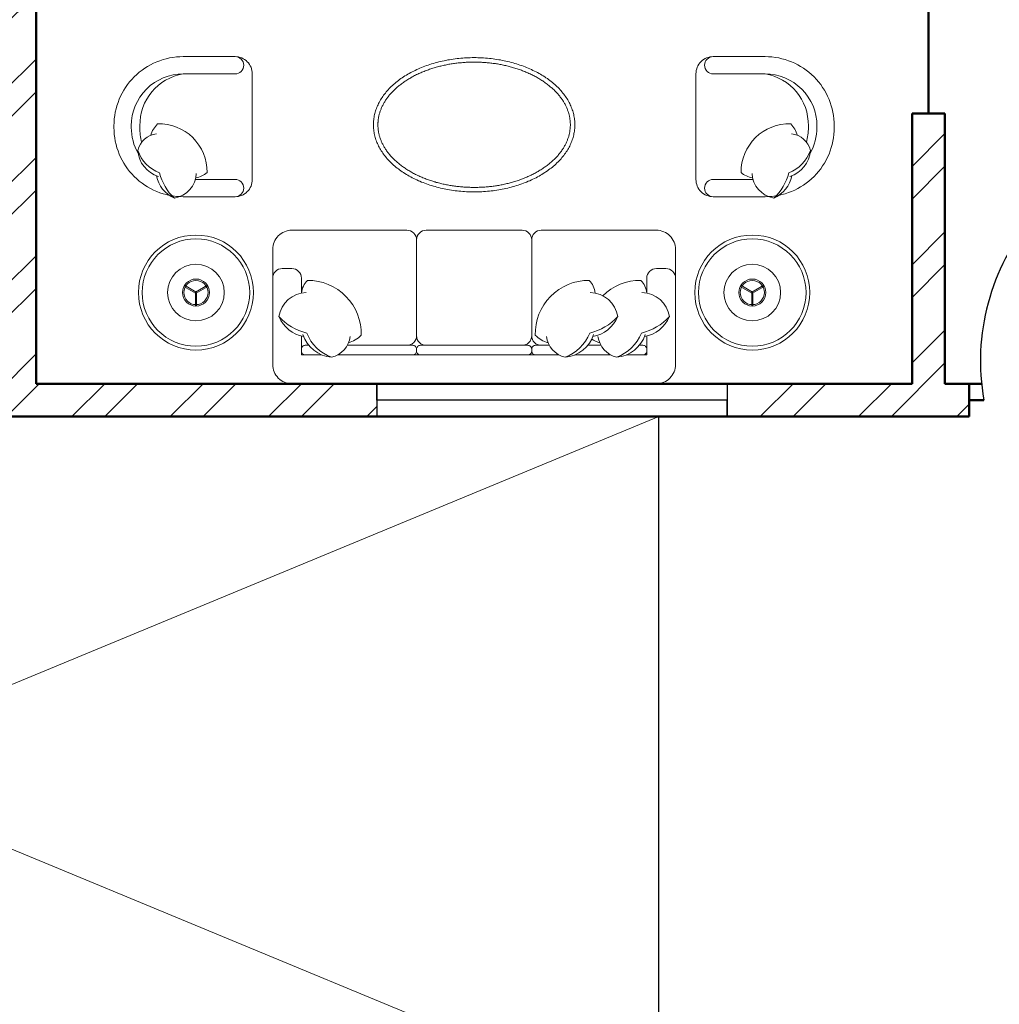
# Model space of a CAD drawing. Units: inches. Extents: x 1901 to 2863, y 888 to 2433.
# Tile 51 of 91: x 2169 to 2303, y 1732 to 1867. Entities that reach past the tile are written whole.
import ezdxf

# ---------------------------------------------------------------- set-up
doc = ezdxf.new("R2010")
doc.units = ezdxf.units.IN
for name, color, linetype, lineweight in [('A-ANNO-SYMB', 8, 'Continuous', 13), ('A-DOOR', 4, 'Continuous', 25), ('A-FLOR-HRAL', 41, 'Continuous', 25), ('A-FURN', 8, 'Continuous', 18), ('A-GLAZ', 3, 'Continuous', 25), ('A-WALL', 7, 'Continuous', 50), ('A-WALL-PATT', 8, 'Continuous', 13)]:
    doc.layers.add(name, color=color, linetype=linetype, lineweight=lineweight)

# ---------------------------------------------------------------- blocks, each defined once
blk = doc.blocks.new('WIN-48')
for p, q in [((0, 2.25), (0, 4.5)), ((0, 4.5), (0, 0)), ((48, 4.5), (48, 0)), ((48, 2.25), (0, 2.25)), ((48, 0), (48, 2.25))]:
    blk.add_line(p, q)

msp = doc.modelspace()

# ---------------------------------------------------------------- hatches: boundary and pattern name
at = {"layer": 'A-WALL-PATT'}
h = msp.add_hatch(dxfattribs=at)
h.set_pattern_fill('ANSI32', color=256)
h.paths.add_polyline_path([(2192.5, 2274.13), (2141.26, 2274.13), (2141.26, 2269.63), (2192.5, 2269.63)])
h.paths.add_polyline_path([(2259.93, 2274.13), (2216.5, 2274.13), (2216.5, 2269.63), (2255.43, 2269.63), (2255.43, 2214.63), (2250.81, 2214.63), (2250.81, 2210.13), (2259.93, 2210.13), (2259.93, 2215.13), (2271.76, 2215.13), (2271.76, 2217.38), (2271.76, 2219.63), (2259.93, 2219.63)])
h.paths.add_polyline_path([(2171.43, 2269.63), (2166.93, 2269.63), (2166.93, 2219.63), (2121.24, 2219.63), (2121.24, 2215.13), (2166.93, 2215.13), (2166.93, 2083.13), (2161.81, 2083.13), (2161.81, 2078.63), (2171.43, 2078.63), (2177, 2078.63), (2177, 2080.88), (2177, 2083.13), (2171.43, 2083.13), (2171.43, 2210.13), (2230.91, 2210.13), (2230.91, 2212.38), (2230.91, 2214.63), (2171.43, 2214.63)])
h.paths.add_polyline_path([(2117.26, 2274.13), (2089.43, 2274.13), (2089.43, 2219.63), (2081.14, 2219.63), (2081.14, 2215.13), (2089.43, 2215.13), (2098, 2215.13), (2098, 2217.38), (2098, 2219.63), (2093.93, 2219.63), (2093.93, 2269.63), (2117.26, 2269.63), (2117.26, 2271.88)])
h.paths.add_polyline_path([(2343.43, 2219.63), (2329.29, 2219.63), (2329.29, 2215.13), (2338.93, 2215.13), (2338.93, 2184.74), (2343.43, 2184.74)])
h.paths.add_polyline_path([(2338.93, 2083.13), (2329.29, 2083.13), (2208.97, 2083.13), (2208.97, 2078.63), (2338.93, 2078.63)])
h.paths.add_polyline_path([(2343.43, 2136.74), (2338.93, 2136.74), (2338.93, 1872.63), (2343.43, 1872.63)])
h.paths.add_polyline_path([(2343.43, 1863.63), (2397.68, 1863.63), (2397.68, 1821.63), (2384.14, 1821.63), (2384.14, 1812.63), (2418.33, 1812.63), (2418.33, 1817.13), (2418.33, 1821.63), (2406.68, 1821.63), (2406.68, 1863.63), (2459.5, 1863.63), (2459.5, 1821.63), (2447.14, 1821.63), (2447.14, 1812.63), (2459.5, 1812.63), (2468.5, 1812.63), (2468.5, 1872.63), (2394.43, 1872.63), (2334.43, 1872.63), (2334.43, 1812.63), (2343.43, 1812.63), (2353.25, 1812.63), (2353.25, 1821.63), (2343.43, 1821.63)])
h.paths.add_polyline_path([(2510.01, 1872.63), (2468.5, 1872.63), (2468.5, 1868.13), (2510.01, 1868.13)])
h.paths.add_polyline_path([(2514.01, 1817.13), (2468.5, 1817.13), (2468.5, 1812.63), (2482.11, 1812.63), (2482.11, 1800.61), (2486.61, 1800.61), (2486.61, 1812.63), (2514.01, 1812.63)])
h.paths.add_polyline_path([(2299.25, 1814.88), (2299.25, 1817.13), (2295.93, 1817.13), (2295.93, 1854.17), (2293.68, 1854.17), (2291.43, 1854.17), (2291.43, 1817.13), (2266.11, 1817.13), (2266.11, 1812.63), (2299.25, 1812.63)])
h.paths.add_polyline_path([(2218.11, 1817.13), (2206.46, 1817.13), (2171.43, 1817.13), (2171.43, 1949.13), (2190.1, 1949.13), (2190.1, 1953.63), (2163.47, 1953.63), (2163.47, 1949.13), (2166.93, 1949.13), (2166.93, 1817.13), (2114.3, 1817.13), (2114.3, 1812.63), (2218.11, 1812.63)])
h.paths.add_polyline_path([(2029.43, 1970.92), (2024.93, 1970.92), (2024.93, 1912.72), (2029.43, 1912.72)])
h.paths.add_polyline_path([(2132.3, 1953.63), (2113.93, 1953.63), (2113.93, 1975.89), (2111.68, 1975.89), (2109.43, 1975.89), (2109.43, 1953.63), (2029.43, 1953.63), (2029.43, 1949.13), (2132.3, 1949.13)])
h.paths.add_polyline_path([(2029.43, 1853.61), (2029.31, 1853.61), (2029.31, 1853.61), (2029.43, 1853.61), (2029.43, 1864.72), (2024.93, 1864.72), (2024.93, 1812.63), (2066.3, 1812.63), (2066.3, 1814.88), (2066.3, 1817.13), (2029.43, 1817.13)])
h.paths.add_polyline_path([(2122.93, 2010.09), (2120.68, 2010.09), (2118.43, 2010.09), (2118.43, 2006.13), (2029.43, 2006.13), (2029.43, 2001.63), (2109.43, 2001.63), (2109.43, 1998.04), (2113.93, 1998.04), (2113.93, 2001.63), (2122.93, 2001.63)])
h.paths.add_polyline_path([(2029.43, 2031.38), (2024.93, 2031.38), (2024.93, 1994.92), (2027.18, 1994.92), (2029.43, 1994.92)])
h.paths.add_polyline_path([(2029.43, 2136.74), (2024.93, 2136.74), (2024.93, 2067.38), (2027.18, 2067.38), (2029.43, 2067.38)])
h.paths.add_polyline_path([(2125.62, 2083.13), (2029.43, 2083.13), (2029.43, 2078.63), (2118.43, 2078.63), (2118.43, 2030.71), (2122.93, 2030.71), (2122.93, 2078.63), (2125.62, 2078.63)])
h.paths.add_polyline_path([(2029.43, 2215.13), (2040.47, 2215.13), (2040.47, 2217.38), (2040.47, 2219.63), (2024.93, 2219.63), (2024.93, 2184.74), (2029.43, 2184.74), (2029.43, 2187.78)])
h.paths.add_polyline_path([(2686.43, 2274.13), (2659.28, 2274.13), (2659.28, 2269.63), (2681.93, 2269.63), (2681.93, 2219.63), (2676.82, 2219.63), (2676.82, 2215.13), (2681.93, 2215.13), (2697.01, 2215.13), (2697.01, 2217.38), (2697.01, 2219.63), (2686.43, 2219.63)])
h.paths.add_polyline_path([(2609.93, 2269.63), (2635.28, 2269.63), (2635.28, 2274.13), (2571.43, 2274.13), (2571.43, 2269.63), (2605.43, 2269.63), (2605.43, 2214.63), (2549.1, 2214.63), (2549.1, 2210.13), (2605.43, 2210.13), (2605.43, 2083.13), (2601.01, 2083.13), (2601.01, 2080.88), (2601.01, 2078.63), (2609.93, 2078.63), (2616.16, 2078.63), (2616.16, 2080.88), (2616.16, 2083.13), (2609.93, 2083.13), (2609.93, 2215.13), (2651.46, 2215.13), (2651.46, 2217.38), (2651.46, 2219.63), (2609.93, 2219.63)])
h.paths.add_polyline_path([(2521.43, 2269.63), (2547.43, 2269.63), (2547.43, 2271.88), (2547.43, 2274.13), (2516.93, 2274.13), (2516.93, 2219.63), (2506.41, 2219.63), (2506.41, 2215.13), (2516.93, 2215.13), (2516.93, 2210.13), (2525.4, 2210.13), (2525.4, 2212.38), (2525.4, 2214.63), (2521.43, 2214.63)])
h.paths.add_polyline_path([(2456.01, 2219.63), (2439.43, 2219.63), (2439.43, 2187.89), (2443.93, 2187.89), (2443.93, 2215.13), (2456.01, 2215.13)])
h.paths.add_polyline_path([(2752.93, 2219.63), (2739.48, 2219.63), (2739.48, 2215.13), (2748.43, 2215.13), (2748.43, 2187.89), (2752.93, 2187.89)])
h.paths.add_polyline_path([(2752.93, 2139.89), (2748.43, 2139.89), (2748.43, 2083.13), (2648.42, 2083.13), (2648.42, 2078.63), (2654.93, 2078.63), (2654.93, 2039.44), (2659.43, 2039.44), (2659.43, 2078.63), (2748.43, 2078.63), (2748.43, 2063.43), (2752.93, 2063.43)])
h.paths.add_polyline_path([(2752.93, 2010.63), (2659.43, 2010.63), (2659.43, 2015.65), (2654.93, 2015.65), (2654.93, 2010.63), (2605.43, 2010.63), (2605.43, 1920.97), (2609.93, 1920.97), (2609.93, 2006.13), (2748.43, 2006.13), (2748.43, 1982.47), (2752.93, 1982.47)])
h.paths.add_polyline_path([(2752.93, 2027.43), (2748.43, 2027.43), (2748.43, 2010.63), (2752.93, 2010.63)])
h.paths.add_polyline_path([(2748.43, 1886.13), (2609.93, 1886.13), (2609.93, 1889.72), (2605.43, 1889.72), (2605.43, 1861.26), (2609.93, 1861.26), (2609.93, 1881.63), (2748.43, 1881.63)])
h.paths.add_polyline_path([(2456.86, 2228.83), (2498.4, 2228.83), (2498.4, 2247.49), (2456.86, 2247.49)], flags=9)
h.paths.add_polyline_path([(2038.6, 2237.42), (2080.17, 2237.42), (2080.17, 2256.08), (2038.6, 2256.08)], flags=9)
h.paths.add_polyline_path([(2292.01, 1062.39), (2539.93, 1062.39), (2539.93, 1099.49), (2292.01, 1099.49)], flags=9)
h.paths.add_polyline_path([(2424.91, 1832.25), (2448.51, 1832.25), (2448.51, 1846.68), (2424.91, 1846.68)], flags=25)
h.paths.add_polyline_path([(2359.08, 1832.25), (2382.68, 1832.25), (2382.68, 1846.68), (2359.08, 1846.68)], flags=25)
h.paths.add_polyline_path([(2352.9, 1684.8), (2367.54, 1684.8), (2367.54, 1697.17), (2352.9, 1697.17)], flags=9)
h.paths.add_polyline_path([(2079.29, 1755.83), (2169.02, 1755.83), (2169.02, 1774.37), (2079.29, 1774.37)], flags=9)
h.paths.add_polyline_path([(2404.09, 1373.86), (2404.09, 1463.59), (2385.54, 1463.59), (2385.54, 1373.86)], flags=9)
h.paths.add_polyline_path([(2268.09, 2236.37), (2309.64, 2236.37), (2309.64, 2255.03), (2268.09, 2255.03)], flags=9)
h.paths.add_polyline_path([(2575.96, 1700.95), (2665.7, 1700.95), (2665.7, 1719.5), (2575.96, 1719.5)], flags=9)
h.paths.add_polyline_path([(2302.96, 1878.47), (2329.52, 1878.47), (2329.52, 1888.78), (2302.96, 1888.78)], flags=9)
h.paths.add_polyline_path([(2097.42, 2240.58), (2126.57, 2240.58), (2126.57, 2259.23), (2097.42, 2259.23)], flags=9)
h.paths.add_polyline_path([(2208.72, 2246.12), (2237.88, 2246.12), (2237.88, 2264.78), (2208.72, 2264.78)], flags=9)
h.paths.add_polyline_path([(2038.15, 1925.96), (2076.99, 1925.96), (2076.99, 1944.62), (2038.15, 1944.62)], flags=9)
h.paths.add_polyline_path([(2239.14, 1926.67), (2288.46, 1926.67), (2288.46, 1945.33), (2239.14, 1945.33)], flags=9)
h.paths.add_polyline_path([(2175.43, 2007.33), (2212.36, 2007.33), (2212.36, 2025.99), (2175.43, 2025.99)], flags=9)
h.paths.add_polyline_path([(2225.03, 2091.79), (2263.87, 2091.79), (2263.87, 2110.45), (2225.03, 2110.45)], flags=9)
h.paths.add_polyline_path([(2035.4, 2098.48), (2074.24, 2098.48), (2074.24, 2117.14), (2035.4, 2117.14)], flags=9)
h.paths.add_polyline_path([(2050.1, 2029.21), (2083.26, 2029.21), (2083.26, 2047.87), (2050.1, 2047.87)], flags=9)
h.paths.add_polyline_path([(2069.68, 1956.72), (2098.83, 1956.72), (2098.83, 1975.38), (2069.68, 1975.38)], flags=25)
h.paths.add_polyline_path([(2328.62, 1753.34), (2361.66, 1753.34), (2361.66, 1771.99), (2328.62, 1771.99)], flags=9)
h.paths.add_polyline_path([(2395.16, 2060.89), (2395.16, 2140.65), (2378.68, 2140.65), (2378.68, 2060.89)], flags=9)
h.paths.add_polyline_path([(2463.73, 2059.02), (2492.89, 2059.02), (2492.89, 2077.68), (2463.73, 2077.68)], flags=9)
h.paths.add_polyline_path([(2458.03, 2181.54), (2496.87, 2181.54), (2496.87, 2200.19), (2458.03, 2200.19)], flags=9)
h.paths.add_polyline_path([(2527.58, 2243.07), (2556.73, 2243.07), (2556.73, 2261.73), (2527.58, 2261.73)], flags=9)
h.paths.add_polyline_path([(2694.46, 2232.77), (2736.03, 2232.77), (2736.03, 2251.42), (2694.46, 2251.42)], flags=9)
h.paths.add_polyline_path([(2637.82, 2249.22), (2666.98, 2249.22), (2666.98, 2267.88), (2637.82, 2267.88)], flags=9)
h.paths.add_polyline_path([(2623.69, 2183.54), (2662.53, 2183.54), (2662.53, 2202.2), (2623.69, 2202.2)], flags=9)
h.paths.add_polyline_path([(2691.97, 2021.5), (2725.12, 2021.5), (2725.12, 2040.16), (2691.97, 2040.16)], flags=9)
h.paths.add_polyline_path([(2621.04, 1975.91), (2662.34, 1975.91), (2662.34, 1994.57), (2621.04, 1994.57)], flags=25)
h.paths.add_polyline_path([(2479.03, 1927.62), (2519.84, 1927.62), (2519.84, 1946.28), (2479.03, 1946.28)], flags=9)
h.paths.add_polyline_path([(2670.94, 1849.08), (2716.01, 1849.08), (2716.01, 1867.73), (2670.94, 1867.73)], flags=9)
h.paths.add_polyline_path([(2523.61, 1782.96), (2550.17, 1782.96), (2550.17, 1793.26), (2523.61, 1793.26)], flags=9)
h.paths.add_polyline_path([(2450.84, 1207.33), (2492.39, 1207.33), (2492.39, 1225.99), (2450.84, 1225.99)], flags=9)
h.paths.add_polyline_path([(2527.75, 1203.84), (2556.91, 1203.84), (2556.91, 1222.5), (2527.75, 1222.5)], flags=9)
h.paths.add_polyline_path([(2639.11, 1207.2), (2668.27, 1207.2), (2668.27, 1225.86), (2639.11, 1225.86)], flags=9)
h.paths.add_polyline_path([(2692.59, 1218.97), (2734.17, 1218.97), (2734.17, 1237.62), (2692.59, 1237.62)], flags=9)
h.paths.add_polyline_path([(2669.27, 1366.33), (2708.11, 1366.33), (2708.11, 1384.99), (2669.27, 1384.99)], flags=9)
h.paths.add_polyline_path([(2463.31, 1358.03), (2502.15, 1358.03), (2502.15, 1376.69), (2463.31, 1376.69)], flags=9)
h.paths.add_polyline_path([(2494.72, 1449.96), (2531.65, 1449.96), (2531.65, 1468.62), (2494.72, 1468.62)], flags=9)
h.paths.add_polyline_path([(2675.57, 1422.16), (2708.72, 1422.16), (2708.72, 1440.81), (2675.57, 1440.81)], flags=9)
h.paths.add_polyline_path([(2685.63, 1493.89), (2714.79, 1493.89), (2714.79, 1512.55), (2685.63, 1512.55)], flags=9)
h.paths.add_polyline_path([(2686.8, 1529.91), (2725.65, 1529.91), (2725.65, 1548.57), (2686.8, 1548.57)], flags=9)
h.paths.add_polyline_path([(2503.65, 1537.99), (2552.97, 1537.99), (2552.97, 1556.65), (2503.65, 1556.65)], flags=9)
h.paths.add_polyline_path([(2291.71, 1643.5), (2318.28, 1643.5), (2318.28, 1653.81), (2291.71, 1653.81)], flags=9)
h.paths.add_polyline_path([(2450.63, 1610.52), (2477.19, 1610.52), (2477.19, 1620.82), (2450.63, 1620.82)], flags=9)
h.paths.add_polyline_path([(2359.99, 1551.81), (2422.25, 1551.81), (2422.25, 1562.12), (2359.99, 1562.12)], flags=9)
h.paths.add_polyline_path([(2280.11, 1249.01), (2321.65, 1249.01), (2321.65, 1267.66), (2280.11, 1267.66)], flags=9)
h.paths.add_polyline_path([(2164.06, 1274.23), (2193.22, 1274.23), (2193.22, 1292.89), (2164.06, 1292.89)], flags=9)
h.paths.add_polyline_path([(2118.21, 1277.69), (2151.25, 1277.69), (2151.25, 1296.35), (2118.21, 1296.35)], flags=9)
h.paths.add_polyline_path([(2031.95, 1268.53), (2073.52, 1268.53), (2073.52, 1287.19), (2031.95, 1287.19)], flags=9)
h.paths.add_polyline_path([(2050.2, 1409.08), (2089.04, 1409.08), (2089.04, 1427.74), (2050.2, 1427.74)], flags=9)
h.paths.add_polyline_path([(2243.74, 1421.03), (2282.58, 1421.03), (2282.58, 1439.69), (2243.74, 1439.69)], flags=9)
h.paths.add_polyline_path([(2190.75, 1509.77), (2231.56, 1509.77), (2231.56, 1528.43), (2190.75, 1528.43)], flags=9)
h.paths.add_polyline_path([(2058.39, 1475.42), (2091.55, 1475.42), (2091.55, 1494.07), (2058.39, 1494.07)], flags=9)
h.paths.add_polyline_path([(2062.45, 1553.09), (2091.6, 1553.09), (2091.6, 1571.75), (2062.45, 1571.75)], flags=9)
h.paths.add_polyline_path([(2219.52, 1590.37), (2266.15, 1590.37), (2266.15, 1609.02), (2219.52, 1609.02)], flags=9)
h.paths.add_polyline_path([(2041.07, 1584.19), (2079.91, 1584.19), (2079.91, 1602.85), (2041.07, 1602.85)], flags=9)

# ---------------------------------------------------------------- linework, layer by layer
at = {"layer": 'A-ANNO-SYMB'}
for p, q in [((2256.71, 1812.63), (2024.93, 1716.63)), ((2024.93, 1812.63), (2256.71, 1716.63))]:
    msp.add_line(p, q, dxfattribs=at)
at = {"layer": 'A-DOOR'}
msp.add_arc((2331.45, 1820.22), 30.67, 90, 190.0141, dxfattribs=at)
at = {"layer": 'A-FLOR-HRAL'}
msp.add_line((2256.71, 1716.63), (2256.71, 1812.63), dxfattribs=at)
at = {"layer": 'A-FURN', "ltscale": 0.03}
for p, q in [((2193.28, 1829.55), (2191.67, 1830.47)), ((2193.36, 1829.69), (2191.76, 1830.61)), ((2193.28, 1829.69), (2194.88, 1830.61)), ((2193.36, 1829.55), (2194.97, 1830.47)), ((2269.49, 1829.55), (2267.89, 1830.47)), ((2269.57, 1829.69), (2267.97, 1830.61)), ((2269.49, 1829.69), (2271.1, 1830.61)), ((2269.57, 1829.55), (2271.18, 1830.47)), ((2193.24, 1829.62), (2193.24, 1827.76)), ((2193.4, 1829.62), (2193.4, 1827.76)), ((2269.45, 1829.62), (2269.45, 1827.76)), ((2269.61, 1829.62), (2269.61, 1827.76))]:
    msp.add_line(p, q, dxfattribs=at)
for points in [[(2201.04, 1852.35), (2201.04, 1859.58, 0.414214), (2198.68, 1861.95), (2191.57, 1861.95, 0.414214), (2182.09, 1852.47), (2182.09, 1852.35), (2182.09, 1852.23, 0.414214), (2191.57, 1842.75), (2198.68, 1842.75, 0.414214), (2201.04, 1845.12), (2201.04, 1852.35)], [(2261.81, 1852.35), (2261.81, 1859.58, -0.414214), (2264.18, 1861.95), (2271.29, 1861.95, -0.414214), (2280.76, 1852.47), (2280.76, 1852.35), (2280.76, 1852.23, -0.414214), (2271.29, 1842.75), (2264.18, 1842.75, -0.414214), (2261.81, 1845.12), (2261.81, 1852.35)]]:
    msp.add_lwpolyline(points, format="xyb", dxfattribs=at)
at = {"layer": 'A-FURN'}
for points in [[(2191.57, 1859.58), (2198.68, 1859.58, 0.414214), (2199.86, 1860.76), (2199.86, 1860.76, 0.414214), (2198.68, 1861.95)], [(2271.29, 1859.58), (2264.18, 1859.58, -0.414214), (2262.99, 1860.76), (2262.99, 1860.76, -0.414214), (2264.18, 1861.95)], [(2191.57, 1859.58, 0.414214), (2184.46, 1852.47), (2184.46, 1852.35)], [(2191.57, 1859.58, 0.372719), (2185.64, 1852.47), (2185.64, 1852.35)], [(2271.29, 1859.58, -0.372719), (2277.21, 1852.47), (2277.21, 1852.35)], [(2271.29, 1859.58, -0.414214), (2278.39, 1852.47), (2278.39, 1852.35)], [(2193.28, 1845.36, 0.165541), (2194.85, 1846.09, 0.425989), (2188.06, 1852.74, 0.121523), (2187.13, 1851.16, -7.115464)], [(2269.57, 1845.36, -0.165541), (2268, 1846.09, -0.425989), (2274.79, 1852.74, -0.121523), (2275.72, 1851.16, 7.115464)], [(2185.4, 1848.7, -0.130591), (2184.46, 1852.23), (2184.46, 1852.35)], [(2188.17, 1845.54, -0.306663), (2185.35, 1849.08, -0.30633), (2187.93, 1851.39, 0.872847)], [(2185.9, 1850.21, -0.072384), (2185.64, 1852.23), (2185.64, 1852.35)], [(2274.68, 1845.54, 0.306663), (2277.5, 1849.08, 0.30633), (2274.92, 1851.39, -0.872847)], [(2276.95, 1850.21, 0.072384), (2277.21, 1852.23), (2277.21, 1852.35)], [(2277.46, 1848.7, 0.130591), (2278.39, 1852.23), (2278.39, 1852.35)], [(2190.37, 1842.56, -0.14773), (2188.33, 1846.02, -0.213343), (2185.35, 1849.08, -0.178662)], [(2272.48, 1842.56, 0.14773), (2274.52, 1846.02, 0.213343), (2277.5, 1849.08, 0.178662)], [(2193.36, 1845.95, -0.356772), (2190.37, 1842.56, -0.249542), (2187.91, 1845.63, 9.61688)], [(2269.5, 1845.95, 0.356772), (2272.48, 1842.56, 0.249542), (2274.94, 1845.63, -9.61688)], [(2193.23, 1845.12), (2198.68, 1845.12, -0.414214), (2199.86, 1843.94), (2199.86, 1843.94, -0.414214), (2198.68, 1842.75)], [(2269.62, 1845.12), (2264.18, 1845.12, 0.414214), (2262.99, 1843.94), (2262.99, 1843.94, 0.414214), (2264.18, 1842.75)], [(2222.23, 1822.39, 0.414214), (2223.54, 1823.7), (2223.54, 1836.84, 0.414214)], [(2240.62, 1822.39, -0.414214), (2239.31, 1823.7), (2239.31, 1836.84, -0.414214)], [(2203.83, 1831.59, -0.414214), (2205.15, 1832.9), (2206.46, 1832.9, -0.414214), (2207.77, 1831.59), (2207.77, 1829.55)], [(2255.08, 1829.55), (2255.08, 1831.59, -0.414214), (2256.39, 1832.9), (2257.71, 1832.9, -0.414214), (2259.02, 1831.59)], [(2207.77, 1829.55, -0.165541), (2208.58, 1831.29, -0.425989), (2215.96, 1823.76, -0.121523), (2214.21, 1822.72, 7.115464)], [(2248, 1829.55, 0.165541), (2247.19, 1831.29, 0.425989), (2239.81, 1823.76, 0.121523), (2241.56, 1822.72, -7.115464)], [(2255.08, 1829.55, 0.165541), (2254.27, 1831.29, 0.200231), (2249.05, 1829.17, 0.121523)], [(2208.43, 1829.63, 0.356772), (2204.67, 1826.32, 0.249542), (2208.08, 1823.59, -9.61688)], [(2247.34, 1829.63, -0.356772), (2251.11, 1826.32, -0.249542), (2247.69, 1823.59, 9.61688)], [(2254.42, 1829.63, -0.356772), (2258.18, 1826.32, -0.249542), (2254.77, 1823.59, 9.61688)], [(2204.67, 1826.32, 0.14773), (2208.51, 1824.06, 0.213343), (2211.9, 1820.75, 0.178662)], [(2251.11, 1826.32, -0.14773), (2247.26, 1824.06, -0.213343), (2243.88, 1820.75, -0.178662)], [(2258.18, 1826.32, -0.14773), (2254.34, 1824.06, -0.213343), (2250.95, 1820.75, -0.178662)], [(2207.98, 1823.88, 0.306663), (2211.9, 1820.75, 0.30633), (2214.46, 1823.61, -0.872847)], [(2224.86, 1822.39, -0.414214), (2223.54, 1823.7)], [(2238, 1822.39, 0.414214), (2239.31, 1823.7)], [(2247.8, 1823.88, -0.306663), (2243.88, 1820.75, -0.30633), (2241.32, 1823.61, 0.872847)], [(2247.54, 1823.24, 0.071865), (2248.64, 1822.72, -7.115464)], [(2254.87, 1823.88, -0.306663), (2250.95, 1820.75, -0.30633), (2248.39, 1823.61, 0.872847)], [(2252.31, 1821.08), (2255.08, 1821.08), (2255.08, 1823.66, -0.414214)], [(2208.78, 1822.39), (2208.3, 1822.39, 0.414214), (2207.77, 1821.86), (2207.77, 1821.6, 0.414214), (2208.3, 1821.08)], [(2212.72, 1821.08), (2223.02, 1821.08, 0.414214), (2223.54, 1821.6), (2223.54, 1821.86, 0.414214), (2223.02, 1822.39), (2214.05, 1822.39, 0.414214)], [(2243.05, 1821.08), (2239.84, 1821.08, -0.414214), (2239.31, 1821.6), (2239.31, 1821.86, -0.414214), (2239.84, 1822.39), (2241.73, 1822.39, -0.414214)], [(2247, 1822.39), (2248.8, 1822.39, -0.414214)], [(2254.08, 1822.39), (2254.55, 1822.39, -0.414214), (2255.08, 1821.86), (2255.08, 1821.6, -0.414214), (2254.55, 1821.08)], [(2208.3, 1821.08), (2210.54, 1821.08, 0.414214)], [(2250.13, 1821.08), (2245.24, 1821.08, -0.414214)], [(2254.55, 1821.08), (2252.31, 1821.08, -0.414214)]]:
    msp.add_lwpolyline(points, format="xyb", dxfattribs=at)
at = {"layer": 'A-FURN', "ltscale": 0.03}
msp.add_lwpolyline([(2203.83, 1835.53, -0.414214), (2206.46, 1838.16), (2222.23, 1838.16, -0.414214), (2223.54, 1836.84, -0.414214), (2224.86, 1838.16), (2238, 1838.16, -0.414214), (2239.31, 1836.84, -0.414214), (2240.62, 1838.16), (2256.39, 1838.16, -0.414214), (2259.02, 1835.53), (2259.02, 1819.76, -0.414214), (2256.39, 1817.13), (2206.46, 1817.13, -0.414214), (2203.83, 1819.76)], format="xyb", close=True, dxfattribs=at)
at = {"layer": 'A-FURN'}
for points in [[(2207.77, 1823.66), (2207.77, 1821.08), (2210.54, 1821.08)], [(2212.72, 1821.08), (2243.05, 1821.08)], [(2245.24, 1821.08), (2250.13, 1821.08)]]:
    msp.add_lwpolyline(points, dxfattribs=at)
msp.add_lwpolyline([(2238.78, 1821.08), (2224.07, 1821.08, -0.414214), (2223.54, 1821.6), (2223.54, 1821.86, -0.414214), (2224.07, 1822.39), (2238.78, 1822.39, -0.414214), (2239.31, 1821.86), (2239.31, 1821.6, -0.414214)], format="xyb", close=True, dxfattribs=at)
at = {"layer": 'A-FURN', "ltscale": 0.03}
msp.add_polyline3d([(2217.63, 1852.61, 0), (2217.63, 1852.44, 0), (2217.64, 1852.26, 0), (2217.65, 1852.09, 0), (2217.67, 1851.92, 0), (2217.69, 1851.74, 0), (2217.72, 1851.57, 0), (2217.75, 1851.4, 0), (2217.79, 1851.22, 0), (2217.83, 1851.05, 0), (2217.88, 1850.88, 0), (2217.93, 1850.71, 0), (2217.98, 1850.54, 0), (2218.04, 1850.37, 0), (2218.11, 1850.2, 0), (2218.18, 1850.04, 0), (2218.26, 1849.87, 0), (2218.34, 1849.7, 0), (2218.42, 1849.54, 0), (2218.51, 1849.38, 0), (2218.61, 1849.21, 0), (2218.7, 1849.05, 0), (2218.81, 1848.89, 0), (2218.92, 1848.73, 0), (2219.03, 1848.58, 0), (2219.14, 1848.42, 0), (2219.27, 1848.27, 0), (2219.39, 1848.11, 0), (2219.52, 1847.96, 0), (2219.66, 1847.81, 0), (2219.79, 1847.67, 0), (2219.94, 1847.52, 0), (2220.08, 1847.38, 0), (2220.23, 1847.23, 0), (2220.39, 1847.09, 0), (2220.55, 1846.95, 0), (2220.71, 1846.82, 0), (2220.88, 1846.68, 0), (2221.05, 1846.55, 0), (2221.22, 1846.42, 0), (2221.4, 1846.3, 0), (2221.58, 1846.17, 0), (2221.76, 1846.05, 0), (2221.95, 1845.93, 0), (2222.14, 1845.81, 0), (2222.34, 1845.69, 0), (2222.54, 1845.58, 0), (2222.74, 1845.47, 0), (2222.94, 1845.36, 0), (2223.15, 1845.25, 0), (2223.36, 1845.15, 0), (2223.57, 1845.05, 0), (2223.79, 1844.95, 0), (2224.01, 1844.86, 0), (2224.23, 1844.76, 0), (2224.45, 1844.68, 0), (2224.68, 1844.59, 0), (2224.91, 1844.5, 0), (2225.14, 1844.42, 0), (2225.37, 1844.35, 0), (2225.61, 1844.27, 0), (2225.85, 1844.2, 0), (2226.09, 1844.13, 0), (2226.33, 1844.06, 0), (2226.57, 1844, 0), (2226.82, 1843.94, 0), (2227.06, 1843.89, 0), (2227.31, 1843.83, 0), (2227.56, 1843.78, 0), (2227.81, 1843.73, 0), (2228.07, 1843.69, 0), (2228.32, 1843.65, 0), (2228.57, 1843.61, 0), (2228.83, 1843.58, 0), (2229.09, 1843.55, 0), (2229.35, 1843.52, 0), (2229.6, 1843.49, 0), (2229.86, 1843.47, 0), (2230.12, 1843.45, 0), (2230.38, 1843.44, 0), (2230.64, 1843.43, 0), (2230.9, 1843.42, 0), (2231.17, 1843.42, 0), (2231.43, 1843.41, 0), (2231.69, 1843.42, 0), (2231.95, 1843.42, 0), (2232.21, 1843.43, 0), (2232.47, 1843.44, 0), (2232.73, 1843.45, 0), (2232.99, 1843.47, 0), (2233.25, 1843.49, 0), (2233.51, 1843.52, 0), (2233.76, 1843.55, 0), (2234.02, 1843.58, 0), (2234.28, 1843.61, 0), (2234.53, 1843.65, 0), (2234.79, 1843.69, 0), (2235.04, 1843.73, 0), (2235.29, 1843.78, 0), (2235.54, 1843.83, 0), (2235.79, 1843.89, 0), (2236.04, 1843.94, 0), (2236.28, 1844, 0), (2236.52, 1844.06, 0), (2236.77, 1844.13, 0), (2237.01, 1844.2, 0), (2237.24, 1844.27, 0), (2237.48, 1844.35, 0), (2237.71, 1844.42, 0), (2237.94, 1844.5, 0), (2238.17, 1844.59, 0), (2238.4, 1844.68, 0), (2238.62, 1844.76, 0), (2238.85, 1844.86, 0), (2239.06, 1844.95, 0), (2239.28, 1845.05, 0), (2239.49, 1845.15, 0), (2239.7, 1845.25, 0), (2239.91, 1845.36, 0), (2240.12, 1845.47, 0), (2240.32, 1845.58, 0), (2240.51, 1845.69, 0), (2240.71, 1845.81, 0), (2240.9, 1845.93, 0), (2241.09, 1846.05, 0), (2241.27, 1846.17, 0), (2241.46, 1846.3, 0), (2241.63, 1846.42, 0), (2241.81, 1846.55, 0), (2241.98, 1846.68, 0), (2242.14, 1846.82, 0), (2242.31, 1846.95, 0), (2242.46, 1847.09, 0), (2242.62, 1847.23, 0), (2242.77, 1847.38, 0), (2242.92, 1847.52, 0), (2243.06, 1847.67, 0), (2243.2, 1847.81, 0), (2243.33, 1847.96, 0), (2243.46, 1848.11, 0), (2243.59, 1848.27, 0), (2243.71, 1848.42, 0), (2243.82, 1848.58, 0), (2243.94, 1848.73, 0), (2244.04, 1848.89, 0), (2244.15, 1849.05, 0), (2244.25, 1849.21, 0), (2244.34, 1849.38, 0), (2244.43, 1849.54, 0), (2244.52, 1849.7, 0), (2244.6, 1849.87, 0), (2244.67, 1850.04, 0), (2244.74, 1850.2, 0), (2244.81, 1850.37, 0), (2244.87, 1850.54, 0), (2244.93, 1850.71, 0), (2244.98, 1850.88, 0), (2245.02, 1851.05, 0), (2245.07, 1851.22, 0), (2245.1, 1851.4, 0), (2245.13, 1851.57, 0), (2245.16, 1851.74, 0), (2245.18, 1851.92, 0), (2245.2, 1852.09, 0), (2245.21, 1852.26, 0), (2245.22, 1852.44, 0), (2245.22, 1852.61, 0), (2245.22, 1852.79, 0), (2245.21, 1852.96, 0), (2245.2, 1853.13, 0), (2245.18, 1853.31, 0), (2245.16, 1853.48, 0), (2245.13, 1853.65, 0), (2245.1, 1853.83, 0), (2245.07, 1854, 0), (2245.02, 1854.17, 0), (2244.98, 1854.34, 0), (2244.93, 1854.51, 0), (2244.87, 1854.68, 0), (2244.81, 1854.85, 0), (2244.74, 1855.02, 0), (2244.67, 1855.19, 0), (2244.6, 1855.35, 0), (2244.52, 1855.52, 0), (2244.43, 1855.68, 0), (2244.34, 1855.85, 0), (2244.25, 1856.01, 0), (2244.15, 1856.17, 0), (2244.04, 1856.33, 0), (2243.94, 1856.49, 0), (2243.82, 1856.65, 0), (2243.71, 1856.8, 0), (2243.59, 1856.96, 0), (2243.46, 1857.11, 0), (2243.33, 1857.26, 0), (2243.2, 1857.41, 0), (2243.06, 1857.56, 0), (2242.92, 1857.7, 0), (2242.77, 1857.85, 0), (2242.62, 1857.99, 0), (2242.46, 1858.13, 0), (2242.31, 1858.27, 0), (2242.14, 1858.4, 0), (2241.98, 1858.54, 0), (2241.81, 1858.67, 0), (2241.63, 1858.8, 0), (2241.46, 1858.93, 0), (2241.27, 1859.05, 0), (2241.09, 1859.18, 0), (2240.9, 1859.3, 0), (2240.71, 1859.42, 0), (2240.51, 1859.53, 0), (2240.32, 1859.65, 0), (2240.12, 1859.76, 0), (2239.91, 1859.86, 0), (2239.7, 1859.97, 0), (2239.49, 1860.07, 0), (2239.28, 1860.17, 0), (2239.06, 1860.27, 0), (2238.85, 1860.37, 0), (2238.62, 1860.46, 0), (2238.4, 1860.55, 0), (2238.17, 1860.63, 0), (2237.94, 1860.72, 0), (2237.71, 1860.8, 0), (2237.48, 1860.88, 0), (2237.24, 1860.95, 0), (2237.01, 1861.02, 0), (2236.77, 1861.09, 0), (2236.52, 1861.16, 0), (2236.28, 1861.22, 0), (2236.04, 1861.28, 0), (2235.79, 1861.34, 0), (2235.54, 1861.39, 0), (2235.29, 1861.44, 0), (2235.04, 1861.49, 0), (2234.79, 1861.53, 0), (2234.53, 1861.57, 0), (2234.28, 1861.61, 0), (2234.02, 1861.65, 0), (2233.76, 1861.68, 0), (2233.51, 1861.7, 0), (2233.25, 1861.73, 0), (2232.99, 1861.75, 0), (2232.73, 1861.77, 0), (2232.47, 1861.78, 0), (2232.21, 1861.79, 0), (2231.95, 1861.8, 0), (2231.69, 1861.81, 0), (2231.43, 1861.81, 0), (2231.17, 1861.81, 0), (2230.9, 1861.8, 0), (2230.64, 1861.79, 0), (2230.38, 1861.78, 0), (2230.12, 1861.77, 0), (2229.86, 1861.75, 0), (2229.6, 1861.73, 0), (2229.35, 1861.7, 0), (2229.09, 1861.68, 0), (2228.83, 1861.65, 0), (2228.57, 1861.61, 0), (2228.32, 1861.57, 0), (2228.07, 1861.53, 0), (2227.81, 1861.49, 0), (2227.56, 1861.44, 0), (2227.31, 1861.39, 0), (2227.06, 1861.34, 0), (2226.82, 1861.28, 0), (2226.57, 1861.22, 0), (2226.33, 1861.16, 0), (2226.09, 1861.09, 0), (2225.85, 1861.02, 0), (2225.61, 1860.95, 0), (2225.37, 1860.88, 0), (2225.14, 1860.8, 0), (2224.91, 1860.72, 0), (2224.68, 1860.63, 0), (2224.45, 1860.55, 0), (2224.23, 1860.46, 0), (2224.01, 1860.37, 0), (2223.79, 1860.27, 0), (2223.57, 1860.17, 0), (2223.36, 1860.07, 0), (2223.15, 1859.97, 0), (2222.94, 1859.86, 0), (2222.74, 1859.76, 0), (2222.54, 1859.65, 0), (2222.34, 1859.53, 0), (2222.14, 1859.42, 0), (2221.95, 1859.3, 0), (2221.76, 1859.18, 0), (2221.58, 1859.05, 0), (2221.4, 1858.93, 0), (2221.22, 1858.8, 0), (2221.05, 1858.67, 0), (2220.88, 1858.54, 0), (2220.71, 1858.4, 0), (2220.55, 1858.27, 0), (2220.39, 1858.13, 0), (2220.23, 1857.99, 0), (2220.08, 1857.85, 0), (2219.94, 1857.7, 0), (2219.79, 1857.56, 0), (2219.66, 1857.41, 0), (2219.52, 1857.26, 0), (2219.39, 1857.11, 0), (2219.27, 1856.96, 0), (2219.14, 1856.8, 0), (2219.03, 1856.65, 0), (2218.92, 1856.49, 0), (2218.81, 1856.33, 0), (2218.7, 1856.17, 0), (2218.61, 1856.01, 0), (2218.51, 1855.85, 0), (2218.42, 1855.68, 0), (2218.34, 1855.52, 0), (2218.26, 1855.35, 0), (2218.18, 1855.19, 0), (2218.11, 1855.02, 0), (2218.04, 1854.85, 0), (2217.98, 1854.68, 0), (2217.93, 1854.51, 0), (2217.88, 1854.34, 0), (2217.83, 1854.17, 0), (2217.79, 1854, 0), (2217.75, 1853.83, 0), (2217.72, 1853.65, 0), (2217.69, 1853.48, 0), (2217.67, 1853.31, 0), (2217.65, 1853.13, 0), (2217.64, 1852.96, 0), (2217.63, 1852.79, 0), (2217.63, 1852.61, 0)], dxfattribs=at)
at = {"layer": 'A-FURN'}
msp.add_polyline3d([(2218.24, 1852.61, 0), (2218.24, 1852.52, 0), (2218.25, 1852.42, 0), (2218.25, 1852.33, 0), (2218.26, 1852.23, 0), (2218.26, 1852.14, 0), (2218.27, 1852.04, 0), (2218.28, 1851.94, 0), (2218.3, 1851.85, 0), (2218.31, 1851.75, 0), (2218.33, 1851.65, 0), (2218.34, 1851.56, 0), (2218.36, 1851.46, 0), (2218.39, 1851.36, 0), (2218.41, 1851.26, 0), (2218.43, 1851.16, 0), (2218.46, 1851.06, 0), (2218.49, 1850.96, 0), (2218.52, 1850.86, 0), (2218.56, 1850.76, 0), (2218.59, 1850.66, 0), (2218.63, 1850.56, 0), (2218.67, 1850.46, 0), (2218.71, 1850.36, 0), (2218.75, 1850.26, 0), (2218.8, 1850.16, 0), (2218.85, 1850.06, 0), (2218.9, 1849.96, 0), (2218.95, 1849.86, 0), (2219, 1849.76, 0), (2219.06, 1849.66, 0), (2219.12, 1849.56, 0), (2219.18, 1849.46, 0), (2219.24, 1849.36, 0), (2219.3, 1849.26, 0), (2219.37, 1849.16, 0), (2219.44, 1849.06, 0), (2219.51, 1848.96, 0), (2219.58, 1848.86, 0), (2219.66, 1848.76, 0), (2219.73, 1848.66, 0), (2219.81, 1848.56, 0), (2219.9, 1848.47, 0), (2219.98, 1848.37, 0), (2220.07, 1848.27, 0), (2220.15, 1848.18, 0), (2220.24, 1848.08, 0), (2220.34, 1847.99, 0), (2220.43, 1847.9, 0), (2220.53, 1847.8, 0), (2220.63, 1847.71, 0), (2220.73, 1847.62, 0), (2220.83, 1847.53, 0), (2220.94, 1847.43, 0), (2221.05, 1847.34, 0), (2221.15, 1847.26, 0), (2221.27, 1847.17, 0), (2221.38, 1847.08, 0), (2221.49, 1846.99, 0), (2221.61, 1846.91, 0), (2221.73, 1846.82, 0), (2221.85, 1846.74, 0), (2221.97, 1846.66, 0), (2222.09, 1846.57, 0), (2222.22, 1846.49, 0), (2222.35, 1846.41, 0), (2222.47, 1846.33, 0), (2222.6, 1846.25, 0), (2222.74, 1846.18, 0), (2222.87, 1846.1, 0), (2223, 1846.03, 0), (2223.14, 1845.95, 0), (2223.28, 1845.88, 0), (2223.41, 1845.81, 0), (2223.55, 1845.74, 0), (2223.7, 1845.67, 0), (2223.84, 1845.6, 0), (2223.98, 1845.54, 0), (2224.13, 1845.47, 0), (2224.27, 1845.41, 0), (2224.42, 1845.35, 0), (2224.57, 1845.29, 0), (2224.72, 1845.23, 0), (2224.87, 1845.17, 0), (2225.02, 1845.12, 0), (2225.17, 1845.06, 0), (2225.32, 1845.01, 0), (2225.48, 1844.96, 0), (2225.63, 1844.91, 0), (2225.78, 1844.86, 0), (2225.94, 1844.81, 0), (2226.09, 1844.77, 0), (2226.24, 1844.72, 0), (2226.4, 1844.68, 0), (2226.55, 1844.64, 0), (2226.71, 1844.6, 0), (2226.86, 1844.56, 0), (2227.02, 1844.52, 0), (2227.18, 1844.49, 0), (2227.33, 1844.45, 0), (2227.49, 1844.42, 0), (2227.65, 1844.39, 0), (2227.8, 1844.36, 0), (2227.96, 1844.33, 0), (2228.12, 1844.3, 0), (2228.28, 1844.27, 0), (2228.44, 1844.25, 0), (2228.59, 1844.23, 0), (2228.75, 1844.2, 0), (2228.91, 1844.18, 0), (2229.07, 1844.16, 0), (2229.23, 1844.15, 0), (2229.39, 1844.13, 0), (2229.55, 1844.11, 0), (2229.71, 1844.1, 0), (2229.87, 1844.09, 0), (2230.03, 1844.07, 0), (2230.19, 1844.06, 0), (2230.35, 1844.06, 0), (2230.51, 1844.05, 0), (2230.67, 1844.04, 0), (2230.83, 1844.04, 0), (2230.99, 1844.03, 0), (2231.15, 1844.03, 0), (2231.31, 1844.03, 0), (2231.47, 1844.03, 0), (2231.63, 1844.03, 0), (2231.79, 1844.03, 0), (2231.95, 1844.03, 0), (2232.11, 1844.04, 0), (2232.27, 1844.04, 0), (2232.43, 1844.05, 0), (2232.59, 1844.06, 0), (2232.75, 1844.07, 0), (2232.91, 1844.08, 0), (2233.07, 1844.09, 0), (2233.22, 1844.11, 0), (2233.38, 1844.12, 0), (2233.54, 1844.14, 0), (2233.7, 1844.15, 0), (2233.86, 1844.17, 0), (2234.02, 1844.19, 0), (2234.18, 1844.21, 0), (2234.34, 1844.24, 0), (2234.5, 1844.26, 0), (2234.65, 1844.29, 0), (2234.81, 1844.31, 0), (2234.97, 1844.34, 0), (2235.13, 1844.37, 0), (2235.28, 1844.4, 0), (2235.44, 1844.43, 0), (2235.6, 1844.47, 0), (2235.75, 1844.5, 0), (2235.91, 1844.54, 0), (2236.07, 1844.58, 0), (2236.22, 1844.62, 0), (2236.38, 1844.66, 0), (2236.53, 1844.7, 0), (2236.69, 1844.74, 0), (2236.84, 1844.79, 0), (2236.99, 1844.84, 0), (2237.15, 1844.88, 0), (2237.3, 1844.93, 0), (2237.45, 1844.98, 0), (2237.61, 1845.04, 0), (2237.76, 1845.09, 0), (2237.91, 1845.14, 0), (2238.06, 1845.2, 0), (2238.21, 1845.26, 0), (2238.36, 1845.32, 0), (2238.51, 1845.38, 0), (2238.65, 1845.44, 0), (2238.8, 1845.51, 0), (2238.94, 1845.57, 0), (2239.09, 1845.64, 0), (2239.23, 1845.71, 0), (2239.37, 1845.78, 0), (2239.51, 1845.85, 0), (2239.64, 1845.92, 0), (2239.78, 1845.99, 0), (2239.92, 1846.06, 0), (2240.05, 1846.14, 0), (2240.18, 1846.22, 0), (2240.31, 1846.29, 0), (2240.44, 1846.37, 0), (2240.57, 1846.45, 0), (2240.7, 1846.53, 0), (2240.82, 1846.61, 0), (2240.94, 1846.7, 0), (2241.06, 1846.78, 0), (2241.18, 1846.86, 0), (2241.3, 1846.95, 0), (2241.42, 1847.04, 0), (2241.53, 1847.12, 0), (2241.64, 1847.21, 0), (2241.75, 1847.3, 0), (2241.86, 1847.39, 0), (2241.97, 1847.48, 0), (2242.07, 1847.57, 0), (2242.17, 1847.66, 0), (2242.27, 1847.76, 0), (2242.37, 1847.85, 0), (2242.47, 1847.94, 0), (2242.56, 1848.04, 0), (2242.65, 1848.13, 0), (2242.74, 1848.23, 0), (2242.83, 1848.32, 0), (2242.92, 1848.42, 0), (2243, 1848.52, 0), (2243.08, 1848.61, 0), (2243.16, 1848.71, 0), (2243.23, 1848.81, 0), (2243.31, 1848.91, 0), (2243.38, 1849.01, 0), (2243.45, 1849.11, 0), (2243.52, 1849.21, 0), (2243.58, 1849.31, 0), (2243.65, 1849.41, 0), (2243.71, 1849.51, 0), (2243.77, 1849.61, 0), (2243.82, 1849.71, 0), (2243.88, 1849.81, 0), (2243.93, 1849.91, 0), (2243.98, 1850.01, 0), (2244.03, 1850.11, 0), (2244.08, 1850.21, 0), (2244.12, 1850.31, 0), (2244.16, 1850.41, 0), (2244.2, 1850.51, 0), (2244.24, 1850.61, 0), (2244.28, 1850.71, 0), (2244.31, 1850.81, 0), (2244.35, 1850.91, 0), (2244.38, 1851.01, 0), (2244.4, 1851.11, 0), (2244.43, 1851.21, 0), (2244.46, 1851.31, 0), (2244.48, 1851.41, 0), (2244.5, 1851.51, 0), (2244.52, 1851.6, 0), (2244.53, 1851.7, 0), (2244.55, 1851.8, 0), (2244.56, 1851.9, 0), (2244.58, 1851.99, 0), (2244.59, 1852.09, 0), (2244.59, 1852.19, 0), (2244.6, 1852.28, 0), (2244.6, 1852.38, 0), (2244.61, 1852.47, 0), (2244.61, 1852.56, 0), (2244.61, 1852.66, 0), (2244.61, 1852.75, 0), (2244.6, 1852.85, 0), (2244.6, 1852.94, 0), (2244.59, 1853.04, 0), (2244.59, 1853.13, 0), (2244.58, 1853.23, 0), (2244.56, 1853.33, 0), (2244.55, 1853.42, 0), (2244.53, 1853.52, 0), (2244.52, 1853.62, 0), (2244.5, 1853.72, 0), (2244.48, 1853.82, 0), (2244.46, 1853.91, 0), (2244.43, 1854.01, 0), (2244.4, 1854.11, 0), (2244.38, 1854.21, 0), (2244.35, 1854.31, 0), (2244.31, 1854.41, 0), (2244.28, 1854.51, 0), (2244.24, 1854.61, 0), (2244.2, 1854.71, 0), (2244.16, 1854.81, 0), (2244.12, 1854.91, 0), (2244.08, 1855.01, 0), (2244.03, 1855.11, 0), (2243.98, 1855.21, 0), (2243.93, 1855.31, 0), (2243.88, 1855.42, 0), (2243.82, 1855.52, 0), (2243.77, 1855.62, 0), (2243.71, 1855.72, 0), (2243.65, 1855.82, 0), (2243.58, 1855.92, 0), (2243.52, 1856.02, 0), (2243.45, 1856.12, 0), (2243.38, 1856.22, 0), (2243.31, 1856.31, 0), (2243.23, 1856.41, 0), (2243.16, 1856.51, 0), (2243.08, 1856.61, 0), (2243, 1856.71, 0), (2242.92, 1856.8, 0), (2242.83, 1856.9, 0), (2242.74, 1857, 0), (2242.65, 1857.09, 0), (2242.56, 1857.19, 0), (2242.47, 1857.28, 0), (2242.37, 1857.38, 0), (2242.27, 1857.47, 0), (2242.17, 1857.56, 0), (2242.07, 1857.65, 0), (2241.97, 1857.74, 0), (2241.86, 1857.83, 0), (2241.75, 1857.92, 0), (2241.64, 1858.01, 0), (2241.53, 1858.1, 0), (2241.42, 1858.19, 0), (2241.3, 1858.27, 0), (2241.18, 1858.36, 0), (2241.06, 1858.44, 0), (2240.94, 1858.53, 0), (2240.82, 1858.61, 0), (2240.7, 1858.69, 0), (2240.57, 1858.77, 0), (2240.44, 1858.85, 0), (2240.31, 1858.93, 0), (2240.18, 1859.01, 0), (2240.05, 1859.08, 0), (2239.92, 1859.16, 0), (2239.78, 1859.23, 0), (2239.64, 1859.31, 0), (2239.51, 1859.38, 0), (2239.37, 1859.45, 0), (2239.23, 1859.52, 0), (2239.09, 1859.59, 0), (2238.94, 1859.65, 0), (2238.8, 1859.72, 0), (2238.65, 1859.78, 0), (2238.51, 1859.84, 0), (2238.36, 1859.9, 0), (2238.21, 1859.96, 0), (2238.06, 1860.02, 0), (2237.91, 1860.08, 0), (2237.76, 1860.13, 0), (2237.61, 1860.19, 0), (2237.45, 1860.24, 0), (2237.3, 1860.29, 0), (2237.15, 1860.34, 0), (2236.99, 1860.39, 0), (2236.84, 1860.43, 0), (2236.69, 1860.48, 0), (2236.53, 1860.52, 0), (2236.38, 1860.57, 0), (2236.22, 1860.61, 0), (2236.07, 1860.65, 0), (2235.91, 1860.68, 0), (2235.75, 1860.72, 0), (2235.6, 1860.75, 0), (2235.44, 1860.79, 0), (2235.28, 1860.82, 0), (2235.13, 1860.85, 0), (2234.97, 1860.88, 0), (2234.81, 1860.91, 0), (2234.65, 1860.94, 0), (2234.5, 1860.96, 0), (2234.34, 1860.99, 0), (2234.18, 1861.01, 0), (2234.02, 1861.03, 0), (2233.86, 1861.05, 0), (2233.7, 1861.07, 0), (2233.54, 1861.09, 0), (2233.38, 1861.1, 0), (2233.22, 1861.12, 0), (2233.07, 1861.13, 0), (2232.91, 1861.14, 0), (2232.75, 1861.15, 0), (2232.59, 1861.16, 0), (2232.43, 1861.17, 0), (2232.27, 1861.18, 0), (2232.11, 1861.19, 0), (2231.95, 1861.19, 0), (2231.79, 1861.19, 0), (2231.63, 1861.2, 0), (2231.47, 1861.2, 0), (2231.31, 1861.2, 0), (2231.15, 1861.19, 0), (2230.99, 1861.19, 0), (2230.83, 1861.19, 0), (2230.67, 1861.18, 0), (2230.51, 1861.18, 0), (2230.35, 1861.17, 0), (2230.19, 1861.16, 0), (2230.03, 1861.15, 0), (2229.87, 1861.14, 0), (2229.71, 1861.12, 0), (2229.55, 1861.11, 0), (2229.39, 1861.09, 0), (2229.23, 1861.08, 0), (2229.07, 1861.06, 0), (2228.91, 1861.04, 0), (2228.75, 1861.02, 0), (2228.59, 1861, 0), (2228.44, 1860.97, 0), (2228.28, 1860.95, 0), (2228.12, 1860.92, 0), (2227.96, 1860.9, 0), (2227.8, 1860.87, 0), (2227.65, 1860.84, 0), (2227.49, 1860.8, 0), (2227.33, 1860.77, 0), (2227.18, 1860.74, 0), (2227.02, 1860.7, 0), (2226.86, 1860.66, 0), (2226.71, 1860.63, 0), (2226.55, 1860.59, 0), (2226.4, 1860.54, 0), (2226.24, 1860.5, 0), (2226.09, 1860.46, 0), (2225.94, 1860.41, 0), (2225.78, 1860.36, 0), (2225.63, 1860.32, 0), (2225.48, 1860.27, 0), (2225.32, 1860.21, 0), (2225.17, 1860.16, 0), (2225.02, 1860.11, 0), (2224.87, 1860.05, 0), (2224.72, 1859.99, 0), (2224.57, 1859.93, 0), (2224.42, 1859.87, 0), (2224.27, 1859.81, 0), (2224.13, 1859.75, 0), (2223.98, 1859.68, 0), (2223.84, 1859.62, 0), (2223.7, 1859.55, 0), (2223.55, 1859.48, 0), (2223.41, 1859.41, 0), (2223.28, 1859.34, 0), (2223.14, 1859.27, 0), (2223, 1859.2, 0), (2222.87, 1859.12, 0), (2222.74, 1859.05, 0), (2222.6, 1858.97, 0), (2222.47, 1858.89, 0), (2222.35, 1858.81, 0), (2222.22, 1858.73, 0), (2222.09, 1858.65, 0), (2221.97, 1858.57, 0), (2221.85, 1858.49, 0), (2221.73, 1858.4, 0), (2221.61, 1858.32, 0), (2221.49, 1858.23, 0), (2221.38, 1858.14, 0), (2221.27, 1858.06, 0), (2221.15, 1857.97, 0), (2221.05, 1857.88, 0), (2220.94, 1857.79, 0), (2220.83, 1857.7, 0), (2220.73, 1857.61, 0), (2220.63, 1857.51, 0), (2220.53, 1857.42, 0), (2220.43, 1857.33, 0), (2220.34, 1857.23, 0), (2220.24, 1857.14, 0), (2220.15, 1857.04, 0), (2220.07, 1856.95, 0), (2219.98, 1856.85, 0), (2219.9, 1856.76, 0), (2219.81, 1856.66, 0), (2219.73, 1856.56, 0), (2219.66, 1856.46, 0), (2219.58, 1856.36, 0), (2219.51, 1856.27, 0), (2219.44, 1856.17, 0), (2219.37, 1856.07, 0), (2219.3, 1855.97, 0), (2219.24, 1855.87, 0), (2219.18, 1855.77, 0), (2219.12, 1855.67, 0), (2219.06, 1855.57, 0), (2219, 1855.47, 0), (2218.95, 1855.37, 0), (2218.9, 1855.26, 0), (2218.85, 1855.16, 0), (2218.8, 1855.06, 0), (2218.75, 1854.96, 0), (2218.71, 1854.86, 0), (2218.67, 1854.76, 0), (2218.63, 1854.66, 0), (2218.59, 1854.56, 0), (2218.56, 1854.46, 0), (2218.52, 1854.36, 0), (2218.49, 1854.26, 0), (2218.46, 1854.16, 0), (2218.43, 1854.06, 0), (2218.41, 1853.96, 0), (2218.39, 1853.86, 0), (2218.36, 1853.77, 0), (2218.34, 1853.67, 0), (2218.33, 1853.57, 0), (2218.31, 1853.47, 0), (2218.3, 1853.38, 0), (2218.28, 1853.28, 0), (2218.27, 1853.18, 0), (2218.26, 1853.09, 0), (2218.26, 1852.99, 0), (2218.25, 1852.9, 0), (2218.25, 1852.8, 0), (2218.24, 1852.71, 0), (2218.24, 1852.61, 0)], dxfattribs=at)
at = {"layer": 'A-FURN', "ltscale": 0.03}
for centre, radius in [((2193.32, 1829.62), 7.88), ((2269.53, 1829.62), 7.88), ((2193.32, 1829.62), 3.88), ((2269.53, 1829.62), 3.88), ((2193.32, 1829.62), 1.85), ((2193.32, 1829.62), 1.66), ((2269.53, 1829.62), 1.85), ((2269.53, 1829.62), 1.66)]:
    msp.add_circle(centre, radius, dxfattribs=at)
at = {"layer": 'A-FURN'}
for centre in [(2193.32, 1829.62), (2269.53, 1829.62)]:
    msp.add_circle(centre, 7.36, dxfattribs=at)
at = {"layer": 'A-WALL'}
for p, q in [((2171.43, 1949.13), (2171.43, 1817.13)), ((2293.68, 1854.17), (2293.68, 1941.24)), ((2291.43, 1854.17), (2295.93, 1854.17)), ((2291.43, 1854.17), (2291.43, 1817.13)), ((2295.93, 1854.17), (2293.68, 1854.17)), ((2295.93, 1854.17), (2295.93, 1817.13)), ((2171.43, 1817.13), (2291.43, 1817.13)), ((2295.93, 1817.13), (2300.93, 1817.13)), ((2299.25, 1817.13), (2299.25, 1812.63)), ((2299.25, 1812.63), (2299.25, 1814.88)), ((2299.25, 1814.88), (2301.25, 1814.88)), ((2024.93, 1812.63), (2299.25, 1812.63))]:
    msp.add_line(p, q, dxfattribs=at)

# ---------------------------------------------------------------- block references
at = {"layer": 'A-GLAZ'}
msp.add_blockref('WIN-48', (2218.11, 1812.63), dxfattribs=at)

doc.saveas('drawing.dxf')
